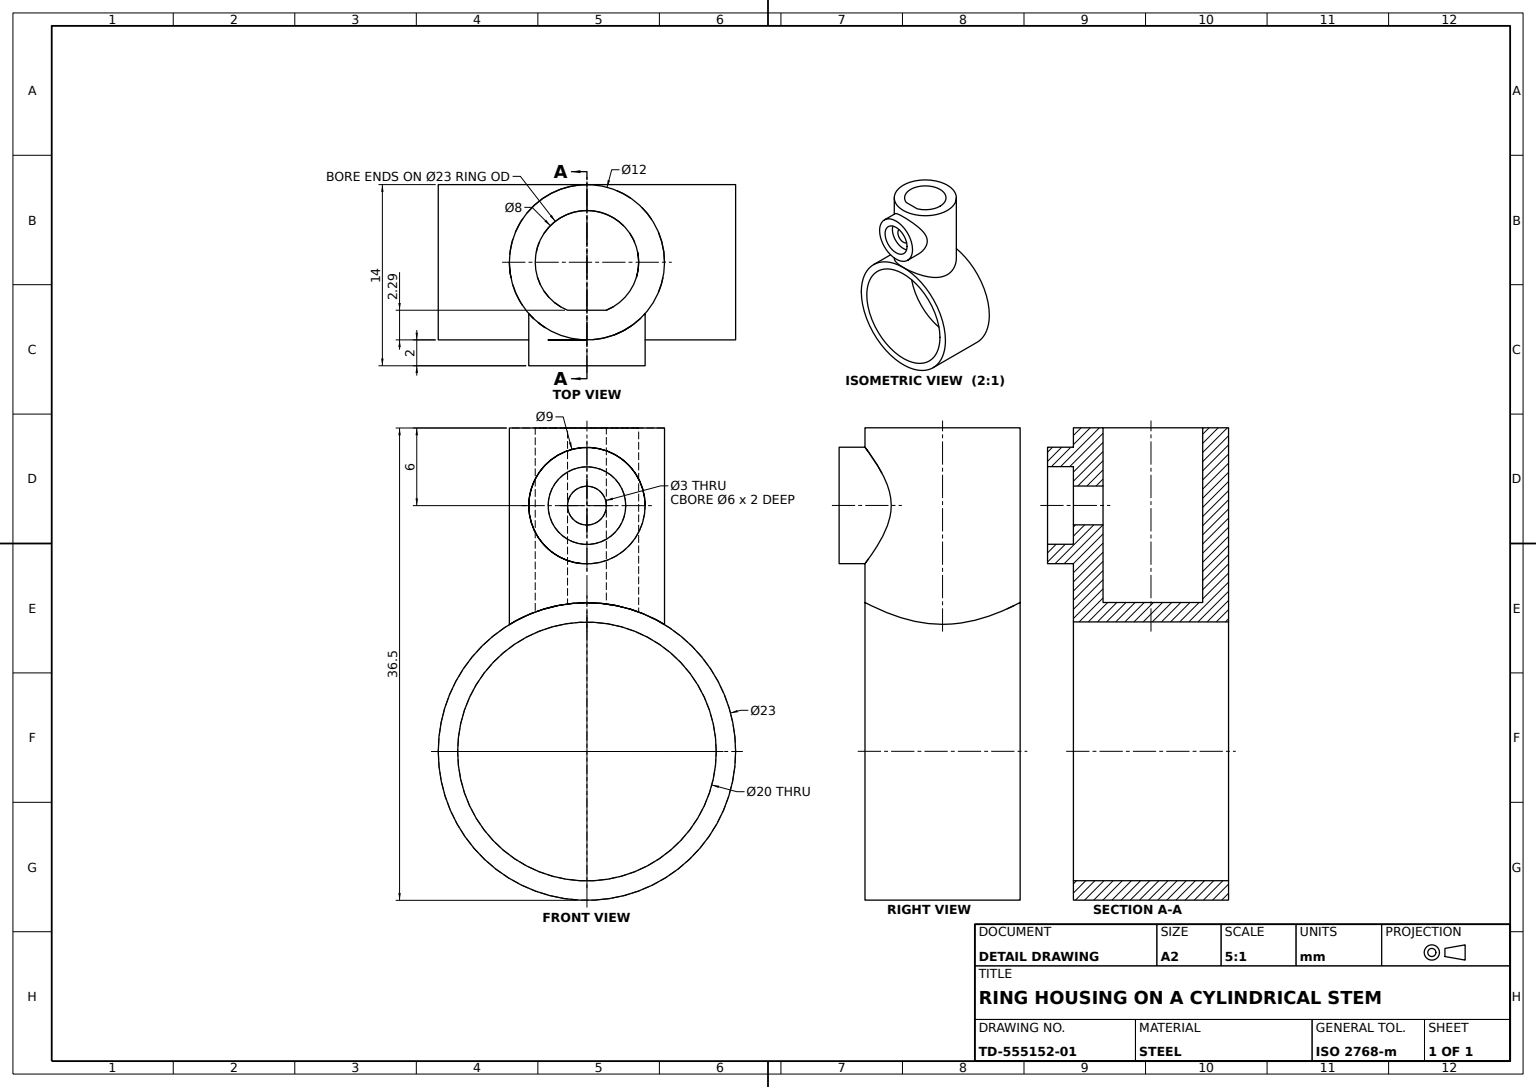
from build123d import *

# Parameters (mm, degrees)
RING_PROFILE_23_20_R      = 11.5
RING_PROFILE_23_20_R_2    = 10
RING_23X12_DEPTH          = 6
STEM_PROFILE_R            = 6
STEM_DEPTH                = 18
RING_START                = -18
RING_CUT_PROFILE_R        = 10
RING_CUT_DEPTH            = 18
SIDE_BOSS_PROFILE_9_R     = 4.5
SIDE_BOSS_9_DEPTH         = 6
SIDE_HOLE_PROFILE_3_R     = 1.5
SIDE_HOLE_3_DEPTH         = 6
COUNTERBORE_PROFILE_6_R   = 3
COUNTERBORE_PROFILE_6_R_2 = 1.5
COUNTERBORE_6X2_DEPTH     = 2
STEM_TRIM_CUT_DEPTH       = 12


with BuildPart() as part:
    # Ring Profile Ø23-Ø20 → Ring Ø23x12 (new, symmetric)
    with BuildSketch(Plane.XY):
        Circle(RING_PROFILE_23_20_R)
        Circle(RING_PROFILE_23_20_R_2, mode=Mode.SUBTRACT)
    extrude(amount=RING_23X12_DEPTH, both=True)

    # Stem Profile → Stem (add)
    with BuildSketch(Plane(origin=(0, -25, 0), x_dir=(-1, 0, 0), z_dir=(0, -1, 0))):
        with Locations(Location((0, 0, 0), (0, 0, 180))):
            Circle(STEM_PROFILE_R)
        with BuildLine():
            Line((-1.5, -3.708099244), (1.5, -3.708099244))
            ThreePointArc((1.5, -3.708099244), (0, 4), (-1.5, -3.708099244))
        make_face(mode=Mode.SUBTRACT)
    extrude(amount=-STEM_DEPTH)

    # Ring Cut Profile → Ring Cut (cut)
    with BuildSketch(Plane.XY.offset(6).offset(RING_START)):
        Circle(RING_CUT_PROFILE_R)
    extrude(amount=RING_CUT_DEPTH, mode=Mode.SUBTRACT)

    # Side Boss Profile Ø9 → Side Boss Ø9 (add)
    with BuildSketch(Plane.XY.offset(8)):
        with Locations((0, -19)):
            Circle(SIDE_BOSS_PROFILE_9_R)
    extrude(amount=-SIDE_BOSS_9_DEPTH)

    # Side Hole Profile Ø3 → Side Hole Ø3 (cut)
    with BuildSketch(Plane.XY.offset(8)):
        with Locations((0, -19)):
            Circle(SIDE_HOLE_PROFILE_3_R)
    extrude(amount=-SIDE_HOLE_3_DEPTH, mode=Mode.SUBTRACT)

    # Counterbore Profile Ø6 → Counterbore Ø6x2 (cut)
    with BuildSketch(Plane.XY.offset(8)):
        with Locations((0, -19)):
            Circle(COUNTERBORE_PROFILE_6_R)
        with Locations((0, -19)):
            Circle(COUNTERBORE_PROFILE_6_R_2, mode=Mode.SUBTRACT)
    extrude(amount=-COUNTERBORE_6X2_DEPTH, mode=Mode.SUBTRACT)

    # Stem Trim Profile → Stem Trim Cut (cut)
    with BuildSketch(Plane.XZ.offset(25)):
        with BuildLine():
            Line((-1.5, 3.708099244), (1.5, 3.708099244))
            ThreePointArc((1.5, 3.708099244), (0, -4), (-1.5, 3.708099244))
        make_face()
    extrude(amount=-STEM_TRIM_CUT_DEPTH, mode=Mode.SUBTRACT)


solid = part.part
